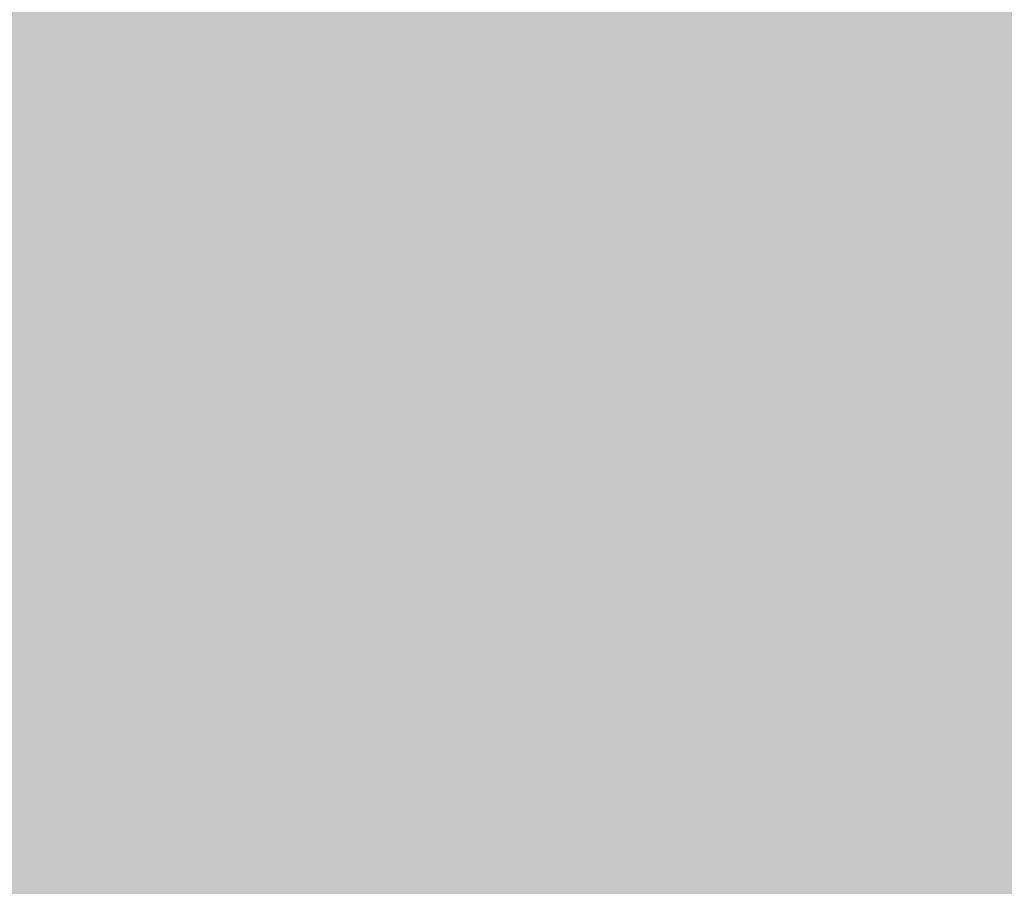
# Model space of a CAD drawing. Units: feet. Extents: x 3168 to 4724, y 827 to 1477.
# Tile 109 of 256: x 3284.48 to 3298.68, y 1074.89 to 1087.4. Entities that reach past the tile are written whole.
import ezdxf

# ---------------------------------------------------------------- set-up
doc = ezdxf.new("R2010")
doc.units = ezdxf.units.FT
doc.layers.add('A-ELEV-PATT', color=8, linetype='Continuous', lineweight=13)

msp = doc.modelspace()

# ---------------------------------------------------------------- hatches: boundary and pattern name
at = {"layer": 'A-ELEV-PATT'}
h = msp.add_hatch(color=256, dxfattribs=at)
h.dxf.hatch_style = 1
edge = h.paths.add_edge_path()
edge.add_ellipse((3552.906, 979.22), major_axis=(36.745, 0), ratio=0.484848, start_angle=0, end_angle=360)
edge = h.paths.add_edge_path()
edge.add_ellipse((3559.892, 929.252), major_axis=(36.745, 0), ratio=0.484848, start_angle=0, end_angle=360)
edge = h.paths.add_edge_path()
edge.add_line((3299.317, 1198.606), (3479.917, 1198.606))
edge.add_line((3479.917, 1198.606), (3479.917, 1209.869))
edge.add_spline(control_points=[(3479.917, 1209.869), (3464.301, 1209.869), (3448.686, 1209.869), (3410.949, 1209.869), (3388.828, 1209.869), (3355.647, 1209.869), (3344.586, 1209.869), (3327.996, 1209.869), (3322.466, 1209.869), (3314.17, 1209.869), (3311.405, 1209.869), (3307.257, 1209.869), (3305.875, 1209.869), (3303.801, 1209.869), (3303.11, 1209.869), (3302.073, 1209.869), (3301.727, 1209.869), (3301.209, 1209.869), (3301.036, 1209.869), (3300.777, 1209.869), (3300.69, 1209.869), (3300.561, 1209.869), (3300.517, 1209.869), (3300.453, 1209.869), (3300.431, 1209.869), (3300.399, 1209.869), (3300.388, 1209.869), (3300.366, 1209.869), (3300.346, 1209.869), (3300.346, 1209.869), (3300.346, 1209.869), (3300.343, 1209.869), (3300.341, 1209.869), (3300.338, 1209.869), (3300.337, 1209.869), (3300.334, 1209.869), (3300.332, 1209.869), (3300.326, 1209.869), (3300.321, 1209.869), (3300.311, 1209.869), (3300.306, 1209.869), (3300.291, 1209.869), (3300.28, 1209.869), (3300.232, 1209.869), (3300.195, 1209.869), (3299.951, 1209.871), (3299.745, 1209.874), (3299.437, 1209.883), (3299.334, 1209.887), (3299.181, 1209.893), (3299.13, 1209.895), (3298.652, 1209.917), (3298.229, 1209.946), (3297.602, 1210.002), (3297.393, 1210.023), (3297.083, 1210.058), (3296.979, 1210.07), (3296.293, 1210.155), (3295.718, 1210.243), (3294.869, 1210.399), (3294.588, 1210.454), (3294.169, 1210.543), (3294.03, 1210.574), (3291.707, 1211.101), (3289.654, 1211.813), (3285.776, 1213.564), (3283.951, 1214.603), (3280.512, 1216.98), (3278.897, 1218.318), (3276.38, 1220.829), (3275.416, 1221.918), (3274.039, 1223.708), (3273.581, 1224.35), (3273.143, 1225.016)], knot_values=[39.119033, 39.119033, 39.119033, 39.119033, 39.286353, 39.286353, 39.523379, 39.523379, 39.641892, 39.641892, 39.701148, 39.701148, 39.730777, 39.730777, 39.745591, 39.745591, 39.752998, 39.752998, 39.756701, 39.756701, 39.758553, 39.758553, 39.759479, 39.759479, 39.759942, 39.759942, 39.760173, 39.760173, 39.760289, 39.760289, 39.760405, 39.760405, 39.760463, 39.760463, 39.763389, 39.763389, 39.764851, 39.764851, 39.767304, 39.767304, 39.773825, 39.773825, 39.78057, 39.78057, 39.79477, 39.79477, 39.845194, 39.845194, 40.126715, 40.126715, 40.267476, 40.267476, 40.337856, 40.337856, 40.927023, 40.927023, 41.221606, 41.221606, 41.368898, 41.368898, 42.202622, 42.202622, 42.619485, 42.619485, 42.827916, 42.827916, 46.118323, 46.118323, 49.408731, 49.408731, 52.699139, 52.699139, 54.927489, 54.927489, 56.104228, 56.104228, 56.104228, 56.104228], weights=[1, 1, 1, 1, 1, 1, 1, 1, 1, 1, 1, 1, 1, 1, 1, 1, 1, 1, 1, 1, 1, 1, 1, 1, 1, 1, 1, 1, 1, 1, 1, 1, 1, 1, 1, 1, 1, 1, 1, 1, 1, 1, 1, 1, 1, 1, 1, 1, 1, 1, 1, 1, 1, 1, 1, 1, 1, 1, 1, 1, 1, 1, 1, 1, 1, 1, 1, 1, 1, 1, 1, 1, 1, 1], degree=3, periodic=0)
edge.add_line((3273.143, 1225.016), (3273.143, 1099.016))
edge.add_line((3273.143, 1099.016), (3299.317, 1099.016))
edge.add_line((3299.317, 1099.016), (3299.317, 1198.606))
edge = h.paths.add_edge_path()
edge.add_line((3304.758, 1324.158), (3479.917, 1324.158))
edge.add_line((3479.917, 1324.158), (3479.917, 1335.715))
edge.add_line((3479.917, 1335.715), (3269.162, 1335.715))
edge.add_spline(control_points=[(3269.162, 1335.715), (3264.024, 1335.715), (3258.364, 1328.958), (3259.264, 1323.9)], knot_values=[0, 0, 0, 0, 15.412191, 15.412191, 15.412191, 15.412191], degree=3, periodic=0)
edge.add_line((3259.264, 1323.9), (3265.517, 1288.769))
edge.add_line((3265.517, 1288.769), (3275.265, 1261.546))
edge.add_line((3275.265, 1261.546), (3304.758, 1261.546))
edge.add_line((3304.758, 1261.546), (3304.758, 1324.158))
h = msp.add_hatch(color=256, dxfattribs=at)
h.dxf.hatch_style = 1
h.paths.add_polyline_path([(3384.525, 1099.016), (3335.029, 1099.016), (3299.317, 1099.016), (3273.143, 1099.016), (3217.565, 1099.016), (3168.069, 827.116), (3335.029, 827.116)])

doc.saveas('drawing.dxf')
